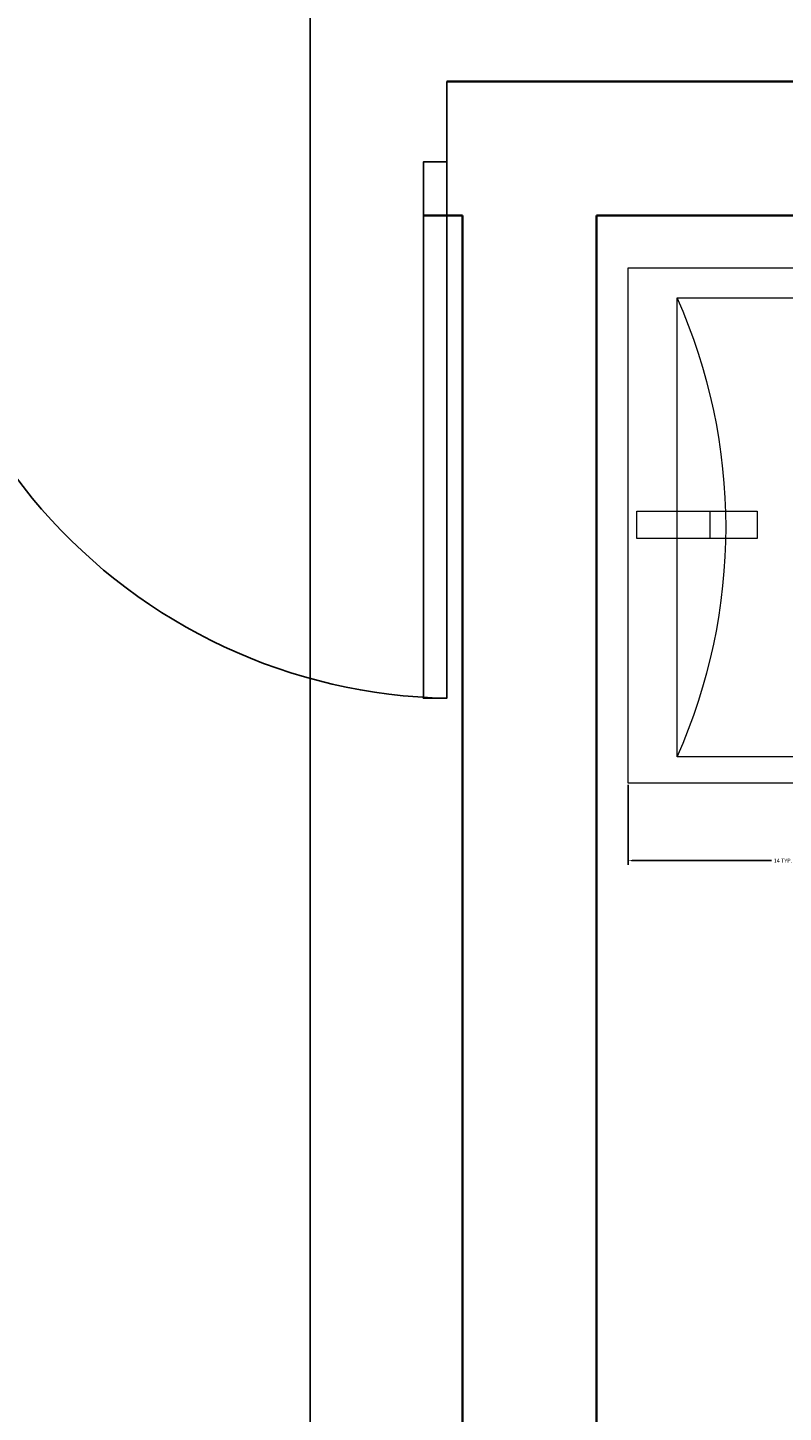
# Model space of a CAD drawing. Units: inches. Extents: x -61 to 1599, y -1316 to 257.
# Tile 86 of 204: x 240 to 274, y -342 to -280. Entities that reach past the tile are written whole.
import ezdxf

# ---------------------------------------------------------------- set-up
doc = ezdxf.new("R2010")
doc.units = ezdxf.units.IN
doc.header["$MEASUREMENT"] = 0
doc.linetypes.add('ACAD_ISO02W100', pattern=[15, 12, -3])
for name, color, linetype, lineweight in [('A-ANNO-DIMS', 2, 'Continuous', 18), ('A-FLOR-FIXT', 8, 'Continuous', 18), ('A-WALL-JAMB', 4, 'ACAD_ISO02W100', 25), ('DOORS', 2, 'Continuous', 25), ('WALLS', 4, 'Continuous', 35)]:
    doc.layers.add(name, color=color, linetype=linetype, lineweight=lineweight)
doc.styles.get("Standard").update_dxf_attribs({"font": 'arial.ttf'})
doc.dimstyles.get("Standard").update_dxf_attribs({"dimtxt": 0.18, "dimasz": 0.18, "dimexe": 0.18, "dimexo": 0.0625, "dimgap": 0.09, "dimtad": 0, "dimtih": 1, "dimtoh": 1, "dimdec": 0, "dimzin": 0, "dimdsep": 46, "dimlunit": 3, "dimtxsty": 'Standard', "dimcen": 0.09, "dimadec": 0, "dimazin": 0, "dimtfac": 1, "dimtdec": 0, "dimtofl": 0, "dimtmove": 0, "dimatfit": 3, "dimfxl": 1, "dimtolj": 1, "dimtzin": 0, "dimarcsym": 0})

# ---------------------------------------------------------------- blocks, each defined once
blk = doc.blocks.new('DOOR-SWING-24')
blk.add_line((0, 0), (0, 3.6))
blk.add_lwpolyline([(0, 0), (0, -24), (1.05, -24), (1.05, 0)], close=True)
blk.add_arc((-0.441, 0.618), 24.622, 271.02591, 6.95592)
blk = doc.blocks.new('LAVATORY-WALL-2')
blk.add_line((3.675, 10.958), (3.675, 12.185))
for points in [[(0, 23.069), (13.865, 23.069), (13.865, 0), (0, 0)], [(12.662, 21.727), (12.662, 1.185), (2.198, 1.185), (2.198, 21.727)], [(5.777, 12.185), (5.777, 10.958), (0.396, 10.958), (0.396, 12.185)]]:
    blk.add_lwpolyline(points, close=True)
for radius in [0.74, 0.233]:
    blk.add_circle((8.705, 11.571), radius)
blk.add_arc((-20.864, 11.456), 25.246, 335.99389, 24.00611)
blk = doc.blocks.new('*D627')
at = {"layer": 'A-ANNO-DIMS', "color": 0, "lineweight": -2, "transparency": 16777216}
for p, q in [((267.117, -313.792), (267.117, -317.37)), ((280.983, -313.792), (280.983, -317.37)), ((267.297, -317.19), (273.53, -317.19)), ((280.803, -317.19), (274.569, -317.19))]:
    blk.add_line(p, q, dxfattribs=at)
at = {"layer": 'A-ANNO-DIMS', "color": 0, "transparency": 16777216}
for points in [[(267.297, -317.16), (267.297, -317.22), (267.117, -317.19)], [(280.803, -317.16), (280.803, -317.22), (280.983, -317.19)]]:
    blk.add_solid(points, dxfattribs=at)
at = {"layer": 'DEFPOINTS', "color": 0, "transparency": 16777216}
for p in [(267.117, -313.73), (280.983, -313.73), (280.983, -317.19)]:
    blk.add_point(p, dxfattribs=at)
at = {"layer": 'A-ANNO-DIMS', "color": 0, "transparency": 16777216, "insert": (274.05, -317.19), "char_height": 0.18, "attachment_point": 5}
blk.add_mtext('\\A1;14 TYP.', dxfattribs=at)
blk = doc.blocks.new('*D687')
at = {"layer": 'A-ANNO-DIMS', "color": 0, "lineweight": -2, "transparency": 16777216}
for p, q in [((289.418, 181.677), (-61.077, 181.677)), ((-60.897, 181.497), (-60.897, -528.952)), ((-60.897, -1239.765), (-60.897, -529.316)), ((319.64, -1239.945), (-61.077, -1239.945))]:
    blk.add_line(p, q, dxfattribs=at)
at = {"layer": 'A-ANNO-DIMS', "color": 0, "transparency": 16777216}
for points in [[(-60.927, 181.497), (-60.867, 181.497), (-60.897, 181.677)], [(-60.927, -1239.765), (-60.867, -1239.765), (-60.897, -1239.945)]]:
    blk.add_solid(points, dxfattribs=at)
at = {"layer": 'DEFPOINTS', "color": 0, "transparency": 16777216}
for p in [(289.481, 181.677), (-60.897, -1239.945), (319.703, -1239.945)]:
    blk.add_point(p, dxfattribs=at)
at = {"layer": 'A-ANNO-DIMS', "color": 0, "transparency": 16777216, "insert": (-60.897, -529.134), "char_height": 0.18, "attachment_point": 5}
blk.add_mtext('\\A1;1421.6', dxfattribs=at)
blk = doc.blocks.new('*D699')
at = {"layer": 'A-ANNO-DIMS', "color": 0, "lineweight": -2, "transparency": 16777216}
for p, q in [((835.64, -167.169), (-61.077, -167.169)), ((-60.897, -167.349), (-60.897, -306.726)), ((-60.897, -446.466), (-60.897, -307.09)), ((841.64, -446.646), (-61.077, -446.646))]:
    blk.add_line(p, q, dxfattribs=at)
at = {"layer": 'A-ANNO-DIMS', "color": 0, "transparency": 16777216}
for points in [[(-60.927, -167.349), (-60.867, -167.349), (-60.897, -167.169)], [(-60.927, -446.466), (-60.867, -446.466), (-60.897, -446.646)]]:
    blk.add_solid(points, dxfattribs=at)
at = {"layer": 'DEFPOINTS', "color": 0, "transparency": 16777216}
for p in [(835.703, -167.169), (-60.897, -446.646), (841.703, -446.646)]:
    blk.add_point(p, dxfattribs=at)
at = {"layer": 'A-ANNO-DIMS', "color": 0, "transparency": 16777216, "insert": (-60.897, -306.908), "char_height": 0.18, "attachment_point": 5}
blk.add_mtext('\\A1;279.5', dxfattribs=at)
blk = doc.blocks.new('*D701')
at = {"layer": 'A-ANNO-DIMS', "color": 0, "lineweight": -2, "transparency": 16777216}
for p, q in [((215.752, -616.882), (215.752, 257.457)), ((215.932, 257.277), (233.924, 257.277)), ((252.702, 257.277), (234.711, 257.277)), ((252.882, -616.882), (252.882, 257.457))]:
    blk.add_line(p, q, dxfattribs=at)
at = {"layer": 'A-ANNO-DIMS', "color": 0, "transparency": 16777216}
for points in [[(215.932, 257.307), (215.932, 257.247), (215.752, 257.277)], [(252.702, 257.307), (252.702, 257.247), (252.882, 257.277)]]:
    blk.add_solid(points, dxfattribs=at)
at = {"layer": 'DEFPOINTS', "color": 0, "transparency": 16777216}
for p in [(252.882, 257.277), (215.752, -616.945), (252.882, -616.945)]:
    blk.add_point(p, dxfattribs=at)
at = {"layer": 'A-ANNO-DIMS', "color": 0, "transparency": 16777216, "insert": (234.317, 257.277), "char_height": 0.18, "attachment_point": 5}
blk.add_mtext('\\A1;37.13', dxfattribs=at)

msp = doc.modelspace()

# ---------------------------------------------------------------- linework, layer by layer
at = {"layer": 'A-WALL-JAMB'}
msp.add_line((258.999, -282.3229), (258.999, -288.3229), dxfattribs=at)
at = {"layer": 'WALLS'}
for p, q in [((258.999, -282.3229), (293.017, -282.3229)), ((257.949, -288.3229), (259.7028, -288.3229)), ((259.7028, -288.3229), (259.7028, -432.3229)), ((265.7028, -288.3229), (265.7028, -367.3229)), ((265.7028, -288.3229), (293.0214, -288.3229))]:
    msp.add_line(p, q, dxfattribs=at)

# ---------------------------------------------------------------- block references
at = {"layer": 'A-FLOR-FIXT'}
msp.add_blockref('LAVATORY-WALL-2', (267.1172, -313.7295), dxfattribs=at)
at = {"layer": 'DOORS', "extrusion": (0, 0, -1), "zscale": -1}
msp.add_blockref('DOOR-SWING-24', (-258.999, -285.9229), dxfattribs=at)

# ---------------------------------------------------------------- dimensions: what is measured, and where the dimension line sits
at = {"layer": 'A-ANNO-DIMS'}
dim = msp.add_linear_dim(base=(252.8825, 257.2771), p1=(215.7521, -616.9446), p2=(252.8825, -616.9446), dimstyle='Standard', override={"dimdec": 2, "dimlfac": 1, "dimrnd": 0, "dimzin": 0, "dimdsep": 46, "dimlunit": 2}, dxfattribs=at)
dim.commit()
dim.dimension.update_dxf_attribs({"geometry": '*D701', "text_midpoint": (234.3173, 257.2771)})
for base, p1, p2, picture, middle in [((-60.8972, -1239.9446), (289.4807, 181.6771), (319.7028, -1239.9446), '*D687', (-60.8972, -529.1337)), ((-60.8972, -446.6462), (835.7028, -167.169), (841.7028, -446.6462), '*D699', (-60.8972, -306.9076))]:
    dim = msp.add_linear_dim(base=base, p1=p1, p2=p2, angle=90, dimstyle='Standard', override={"dimdec": 1, "dimlfac": 1, "dimrnd": 0, "dimzin": 0, "dimdsep": 46, "dimlunit": 2}, dxfattribs=at)
    dim.commit()
    dim.dimension.update_dxf_attribs({"geometry": picture, "text_midpoint": middle})
dim = msp.add_linear_dim(base=(280.9827, -317.1903), p1=(267.117, -313.73), p2=(280.9827, -313.73), text='<> TYP.', dimstyle='Standard', override={"dimdec": 0, "dimlfac": 1, "dimrnd": 0, "dimzin": 0, "dimdsep": 46, "dimlunit": 2}, dxfattribs=at)
dim.commit()
dim.dimension.update_dxf_attribs({"geometry": '*D627', "text_midpoint": (274.0498, -317.1903)})

doc.saveas('drawing.dxf')
